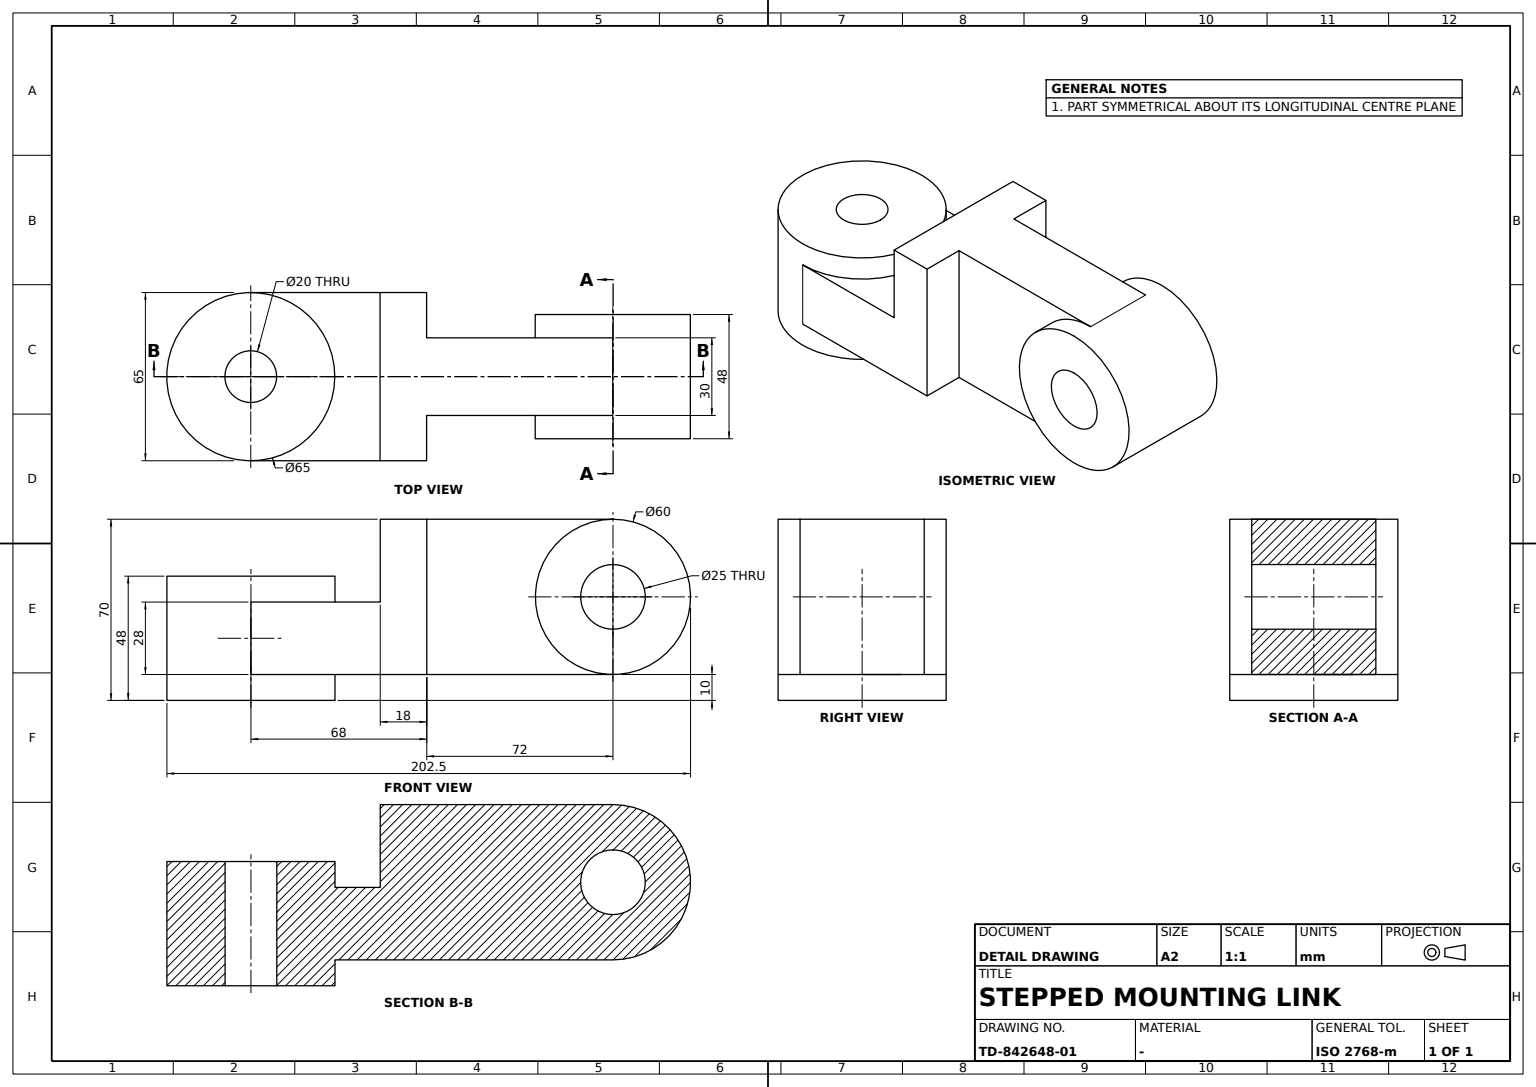
CATIA V5 part; units mm, degrees
sketch "Sketch1" plane through (0, 0, 0) normal (0, 0, 1) x (1, 0, 0)
  line L0 (34, 32.5) -> (34, -32.5)
  line L1 (34, -32.5) -> (-34, -32.5)
  line L2 (-34, -32.5) -> (-34, 32.5)
  line L3 (-34, 32.5) -> (34, 32.5)
  dimension "distance L1 L3" = 65
  dimension "distance L0 L2" = 68
  constraint vertical L0 y-axis
  constraint vertical L2 y-axis
  constraint horizontal L1 x-axis
  constraint horizontal L3 x-axis
  constraint equidistance L0 L2 origin
  constraint equidistance L1 L3 origin
extrude "Pad1" add sketch "Sketch1" along normal blind 28
sketch "Sketch2" plane through (0, 0, 28) normal (0, 0, 1) x (1, 0, 0)
  line L0 (34, 32.5) -> (16, 32.5)
  line L1 (16, 32.5) -> (16, -32.5)
  line L2 (16, -32.5) -> (34, -32.5)
  line L3 (34, 32.5) -> (34, -32.5)
  dimension "length L0" = 18
  constraint horizontal L0 x-axis
  constraint horizontal L2 x-axis
  constraint vertical L1 y-axis
  constraint vertical L3 y-axis
extrude "Pad2" add sketch "Sketch2" along normal blind 32
sketch "Sketch3" plane through (0, 0, 60) normal (0, 0, 1) x (1, 0, 0)
  point P0 (34, 0)
  line L0 (106, 15) -> (34, 15)
  line L1 (34, 15) -> (34, -15)
  line L2 (34, -15) -> (106, -15)
  line L3 (106, -15) -> (106, 15)
  dimension "length L1" = 30
  constraint horizontal L0 x-axis
  constraint horizontal L2 x-axis
  constraint vertical L1 y-axis
  constraint vertical L3 y-axis
extrude "Pad3" add sketch "Sketch3" against normal blind 60
ref_plane "Plane1" through (0, 0, 14) normal (0, 0, 1) x (1, 0, 0)
sketch "Sketch4" plane through (0, 0, 14) normal (0, 0, 1) x (1, 0, 0)
  circle A0 centre (-34, 0) radius 32.5
  point P0 (-34, 0)
  line L0 (34, -32.5) -> (34, 32.5) construction
  dimension "radius A0" = 32.5
  dimension "distance P0 L0" = 68
  constraint coincidence P0 x-axis
extrude "Pad4" add sketch "Sketch4" along normal mid plane 48
sketch "Sketch5" plane through (0, 0, 38) normal (0, 0, 1) x (1, 0, 0)
  circle A0 centre (-34, 0) radius 10
  point P0 (-34, 0)
  line L0 (34, -32.5) -> (34, 32.5) construction
  dimension "radius A0" = 10
  dimension "distance P0 L0" = 68
  constraint coincidence P0 x-axis
extrude "Pocket1" cut sketch "Sketch5" against normal blind 48
sketch "Sketch6" plane through (0, 0, 0) normal (0, 1, 0) x (-1, 0, 0)
  point P0 (-106, 0)
  circle A0 centre (-106, 30) radius 30
  point P1 (-106, 30)
  dimension "radius A0" = 30
  dimension "distance P1 P0" = 30
extrude "Pad5" add sketch "Sketch6" along normal mid plane 48
sketch "Sketch7" plane through (0, -24, 0) normal (0, -1, 0) x (1, 0, 0)
  circle A0 centre (106, 30) radius 12.5
  point P0 (106, 30)
  line L0 (34, 0) -> (34, 28) construction
  line L1 (34, 0) -> (106, 0) construction
  dimension "radius A0" = 12.5
  dimension "distance P0 L0" = 72
  dimension "distance P0 L1" = 30
extrude "Pocket2" cut sketch "Sketch7" against normal blind 48
